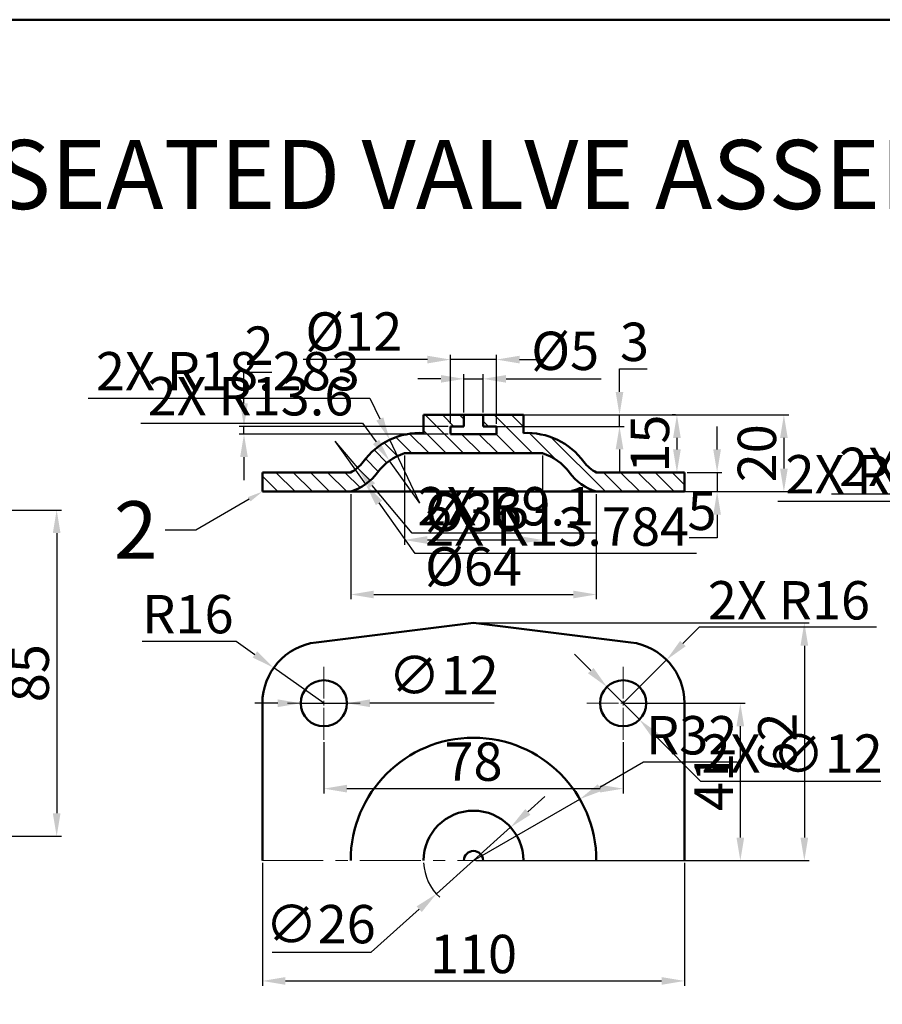
# Model space of a CAD drawing. Units: millimetres. Extents: x 147 to 984, y -369 to 435.
# Tile 7 of 10: x 475 to 699, y 179 to 435. Entities that reach past the tile are written whole.
import ezdxf
from ezdxf import colors
from ezdxf.entities.mleader import LeaderData, LeaderLine
from ezdxf.math import Vec2, Vec3

# ---------------------------------------------------------------- set-up
doc = ezdxf.new("R2010")
doc.units = ezdxf.units.MM
doc.header["$LTSCALE"] = 0.5
doc.linetypes.add('CENTER', pattern=[50.8, 31.75, -6.35, 6.35, -6.35])
for name, color, linetype, lineweight in [('M-CNTR', 1, 'CENTER', 18), ('M-DIMS', 2, 'Continuous', 25), ('M-HATC', 8, 'Continuous', 18), ('M-OUTL', 7, 'Continuous', 50), ('M-TEXT', 7, 'Continuous', 25)]:
    doc.layers.add(name, color=color, linetype=linetype, lineweight=lineweight)
doc.styles.get("Standard").update_dxf_attribs({"font": 'arial.ttf'})
doc.dimstyles.new('ISO-25', dxfattribs={"dimtxt": 10, "dimasz": 6, "dimexe": 1.25, "dimexo": 0.625, "dimtad": 1, "dimtoh": 1, "dimdec": 0, "dimtxsty": 'Standard', "dimcen": 2.5, "dimadec": 0, "dimazin": 0, "dimtfac": 1, "dimtdec": 0, "dimtmove": 0, "dimatfit": 3, "dimfxl": 1, "dimarcsym": 0})

# ---------------------------------------------------------------- blocks, each defined once
blk = doc.blocks.new('*D2')
at = {"layer": 'Defpoints', "color": 0, "transparency": 16777216}
for p in [(439.82, 307.49), (439.82, 222.49), (484.37, 222.49)]:
    blk.add_point(p, dxfattribs=at)
at = {"layer": 'M-DIMS', "color": 0, "lineweight": -2, "transparency": 16777216}
for p, q in [((440.44, 307.49), (485.62, 307.49)), ((484.37, 301.49), (484.37, 228.49)), ((440.44, 222.49), (485.62, 222.49))]:
    blk.add_line(p, q, dxfattribs=at)
at = {"layer": 'M-DIMS', "color": 0, "transparency": 16777216}
for points in [[(483.37, 301.49), (485.37, 301.49), (484.37, 307.49)], [(483.37, 228.49), (485.37, 228.49), (484.37, 222.49)]]:
    blk.add_solid(points, dxfattribs=at)
at = {"layer": 'M-DIMS', "color": 0, "transparency": 16777216, "insert": (478.64, 264.99), "char_height": 10, "attachment_point": 5, "rotation": 90}
blk.add_mtext('85', dxfattribs=at)
blk = doc.blocks.new('*U27')
at = {"layer": 'M-CNTR', "color": 0, "transparency": 16777216}
for p, q in [((0, 1.2), (0, 9.5)), ((-9.5, 0), (-1.2, 0)), ((1.2, 0), (9.5, 0)), ((0, -9.5), (0, -1.2))]:
    blk.add_line(p, q, dxfattribs=at)
at = {"layer": 'M-CNTR', "color": 0, "linetype": 'Continuous', "transparency": 16777216}
for p, q in [((-0.6, 0), (0.6, 0)), ((0, -0.6), (0, 0.6))]:
    blk.add_line(p, q, dxfattribs=at)
blk = doc.blocks.new('*U28')
at = {"layer": 'M-CNTR', "color": 0, "transparency": 16777216}
for p, q in [((0, 1.2), (0, 9.5)), ((-9.5, 0), (-1.2, 0)), ((1.2, 0), (9.5, 0)), ((0, -9.5), (0, -1.2))]:
    blk.add_line(p, q, dxfattribs=at)
at = {"layer": 'M-CNTR', "color": 0, "linetype": 'Continuous', "transparency": 16777216}
for p, q in [((-0.6, 0), (0.6, 0)), ((0, -0.6), (0, 0.6))]:
    blk.add_line(p, q, dxfattribs=at)
blk = doc.blocks.new('*D29')
at = {"layer": 'Defpoints', "color": 0, "transparency": 16777216}
for p in [(595.47, 341.7), (590.47, 332.31), (595.47, 332.31)]:
    blk.add_point(p, dxfattribs=at)
at = {"layer": 'M-DIMS', "color": 0, "lineweight": -2, "transparency": 16777216}
for p, q in [((584.47, 341.7), (578.47, 341.7)), ((590.47, 332.94), (590.47, 342.95)), ((590.47, 341.7), (595.47, 341.7)), ((595.47, 332.94), (595.47, 342.95)), ((601.47, 341.7), (626.23, 341.7))]:
    blk.add_line(p, q, dxfattribs=at)
at = {"layer": 'M-DIMS', "color": 0, "transparency": 16777216}
for points in [[(584.47, 342.7), (584.47, 340.7), (590.47, 341.7)], [(601.47, 342.7), (601.47, 340.7), (595.47, 341.7)]]:
    blk.add_solid(points, dxfattribs=at)
at = {"layer": 'M-DIMS', "color": 0, "transparency": 16777216, "insert": (616.85, 347.71), "char_height": 10, "attachment_point": 5}
blk.add_mtext('%%C5', dxfattribs=at)
blk = doc.blocks.new('*D30')
at = {"layer": 'Defpoints', "color": 0, "transparency": 16777216}
for p in [(598.97, 346.73), (586.97, 329.31), (598.97, 329.31)]:
    blk.add_point(p, dxfattribs=at)
at = {"layer": 'M-DIMS', "color": 0, "lineweight": -2, "transparency": 16777216}
for p, q in [((580.97, 346.73), (548.62, 346.73)), ((586.97, 329.94), (586.97, 347.98)), ((598.97, 346.73), (586.97, 346.73)), ((598.97, 329.94), (598.97, 347.98)), ((604.97, 346.73), (610.97, 346.73))]:
    blk.add_line(p, q, dxfattribs=at)
at = {"layer": 'M-DIMS', "color": 0, "transparency": 16777216}
for points in [[(580.97, 347.73), (580.97, 345.73), (586.97, 346.73)], [(604.97, 347.73), (604.97, 345.73), (598.97, 346.73)]]:
    blk.add_solid(points, dxfattribs=at)
at = {"layer": 'M-DIMS', "color": 0, "transparency": 16777216, "insert": (561.79, 352.74), "char_height": 10, "attachment_point": 5}
blk.add_mtext('%%C12', dxfattribs=at)
blk = doc.blocks.new('*D31')
at = {"layer": 'Defpoints', "color": 0, "transparency": 16777216}
for p in [(595.47, 332.31), (595.47, 329.31), (631.01, 329.31)]:
    blk.add_point(p, dxfattribs=at)
at = {"layer": 'M-DIMS', "color": 0, "lineweight": -2, "transparency": 16777216}
for p, q in [((631.01, 338.31), (631.01, 344.31)), ((631.01, 344.31), (638.18, 344.31)), ((596.1, 332.31), (632.26, 332.31)), ((631.01, 329.31), (631.01, 332.31)), ((596.1, 329.31), (632.26, 329.31)), ((631.01, 323.31), (631.01, 317.31))]:
    blk.add_line(p, q, dxfattribs=at)
at = {"layer": 'M-DIMS', "color": 0, "transparency": 16777216}
for points in [[(630.01, 338.31), (632.01, 338.31), (631.01, 332.31)], [(630.01, 323.31), (632.01, 323.31), (631.01, 329.31)]]:
    blk.add_solid(points, dxfattribs=at)
at = {"layer": 'M-DIMS', "color": 0, "transparency": 16777216, "insert": (634.91, 350.05), "char_height": 10, "attachment_point": 5}
blk.add_mtext('3', dxfattribs=at)
blk = doc.blocks.new('*D32')
at = {"layer": 'Defpoints', "color": 0, "transparency": 16777216}
for p in [(586.97, 329.31), (533.17, 327.31), (586.97, 327.31)]:
    blk.add_point(p, dxfattribs=at)
at = {"layer": 'M-DIMS', "color": 0, "lineweight": -2, "transparency": 16777216}
for p, q in [((533.17, 335.31), (533.17, 343.41)), ((533.17, 343.41), (540.42, 343.41)), ((586.35, 329.31), (531.92, 329.31)), ((533.17, 327.31), (533.17, 329.31)), ((586.35, 327.31), (531.92, 327.31)), ((533.17, 321.31), (533.17, 315.31))]:
    blk.add_line(p, q, dxfattribs=at)
at = {"layer": 'M-DIMS', "color": 0, "transparency": 16777216}
for points in [[(532.17, 335.31), (534.17, 335.31), (533.17, 329.31)], [(532.17, 321.31), (534.17, 321.31), (533.17, 327.31)]]:
    blk.add_solid(points, dxfattribs=at)
at = {"layer": 'M-DIMS', "color": 0, "transparency": 16777216, "insert": (537.11, 349.06), "char_height": 10, "attachment_point": 5}
blk.add_mtext('2', dxfattribs=at)
blk = doc.blocks.new('*D33')
at = {"layer": 'Defpoints', "color": 0, "transparency": 16777216}
for p in [(560.97, 312.31), (624.97, 312.31), (624.97, 285.51)]:
    blk.add_point(p, dxfattribs=at)
at = {"layer": 'M-DIMS', "color": 0, "lineweight": -2, "transparency": 16777216}
for p, q in [((560.97, 311.69), (560.97, 284.26)), ((624.97, 311.69), (624.97, 284.26)), ((566.97, 285.51), (618.97, 285.51))]:
    blk.add_line(p, q, dxfattribs=at)
at = {"layer": 'M-DIMS', "color": 0, "transparency": 16777216}
for points in [[(566.97, 286.51), (566.97, 284.51), (560.97, 285.51)], [(618.97, 286.51), (618.97, 284.51), (624.97, 285.51)]]:
    blk.add_solid(points, dxfattribs=at)
at = {"layer": 'M-DIMS', "color": 0, "transparency": 16777216, "insert": (592.97, 291.52), "char_height": 10, "attachment_point": 5}
blk.add_mtext('%%C64', dxfattribs=at)
blk = doc.blocks.new('*D34')
at = {"layer": 'Defpoints', "color": 0, "transparency": 16777216}
for p in [(574.97, 322.31), (610.97, 322.31), (610.97, 299.71)]:
    blk.add_point(p, dxfattribs=at)
at = {"layer": 'M-DIMS', "color": 0, "lineweight": -2, "transparency": 16777216}
for p, q in [((574.97, 321.69), (574.97, 298.46)), ((610.97, 321.69), (610.97, 298.46)), ((580.97, 299.71), (604.97, 299.71))]:
    blk.add_line(p, q, dxfattribs=at)
at = {"layer": 'M-DIMS', "color": 0, "transparency": 16777216}
for points in [[(580.97, 300.71), (580.97, 298.71), (574.97, 299.71)], [(604.97, 300.71), (604.97, 298.71), (610.97, 299.71)]]:
    blk.add_solid(points, dxfattribs=at)
at = {"layer": 'M-DIMS', "color": 0, "transparency": 16777216, "insert": (592.97, 305.72), "char_height": 10, "attachment_point": 5}
blk.add_mtext('%%C36', dxfattribs=at)
blk = doc.blocks.new('*D35')
at = {"layer": 'Defpoints', "color": 0, "transparency": 16777216}
for p in [(593.07, 332.31), (592.97, 312.31), (673.84, 312.31)]:
    blk.add_point(p, dxfattribs=at)
at = {"layer": 'M-DIMS', "color": 0, "lineweight": -2, "transparency": 16777216}
for p, q in [((593.69, 332.31), (675.09, 332.31)), ((673.84, 326.31), (673.84, 318.31)), ((593.6, 312.31), (675.09, 312.31))]:
    blk.add_line(p, q, dxfattribs=at)
at = {"layer": 'M-DIMS', "color": 0, "transparency": 16777216}
for points in [[(672.84, 326.31), (674.84, 326.31), (673.84, 332.31)], [(672.84, 318.31), (674.84, 318.31), (673.84, 312.31)]]:
    blk.add_solid(points, dxfattribs=at)
at = {"layer": 'M-DIMS', "color": 0, "transparency": 16777216, "insert": (668.1, 322.31), "char_height": 10, "attachment_point": 5, "rotation": 90}
blk.add_mtext('20', dxfattribs=at)
blk = doc.blocks.new('*D36')
at = {"layer": 'Defpoints', "color": 0, "transparency": 16777216}
for p in [(647.97, 317.31), (647.97, 312.31), (656.44, 312.31)]:
    blk.add_point(p, dxfattribs=at)
at = {"layer": 'M-DIMS', "color": 0, "lineweight": -2, "transparency": 16777216}
for p, q in [((656.44, 323.31), (656.44, 329.31)), ((648.6, 317.31), (657.69, 317.31)), ((656.44, 317.31), (656.44, 312.31)), ((648.6, 312.31), (657.69, 312.31)), ((656.44, 306.31), (656.44, 300.31)), ((656.44, 300.31), (649.19, 300.31))]:
    blk.add_line(p, q, dxfattribs=at)
at = {"layer": 'M-DIMS', "color": 0, "transparency": 16777216}
for points in [[(655.44, 323.31), (657.44, 323.31), (656.44, 317.31)], [(655.44, 306.31), (657.44, 306.31), (656.44, 312.31)]]:
    blk.add_solid(points, dxfattribs=at)
at = {"layer": 'M-DIMS', "color": 0, "transparency": 16777216, "insert": (652.5, 306.02), "char_height": 10, "attachment_point": 5}
blk.add_mtext('5', dxfattribs=at)
blk = doc.blocks.new('*D37')
at = {"layer": 'Defpoints', "color": 0, "transparency": 16777216}
for p in [(646.27, 332.31), (645.97, 317.31), (646.27, 317.31)]:
    blk.add_point(p, dxfattribs=at)
at = {"layer": 'M-DIMS', "color": 0, "lineweight": -2, "transparency": 16777216}
for p, q in [((645.64, 332.31), (644.72, 332.31)), ((645.97, 326.31), (645.97, 323.31)), ((645.64, 317.31), (644.72, 317.31))]:
    blk.add_line(p, q, dxfattribs=at)
at = {"layer": 'M-DIMS', "color": 0, "transparency": 16777216}
for points in [[(644.97, 326.31), (646.97, 326.31), (645.97, 332.31)], [(644.97, 323.31), (646.97, 323.31), (645.97, 317.31)]]:
    blk.add_solid(points, dxfattribs=at)
at = {"layer": 'M-DIMS', "color": 0, "transparency": 16777216, "insert": (640.24, 324.81), "char_height": 10, "attachment_point": 5, "rotation": 90}
blk.add_mtext('15', dxfattribs=at)
blk = doc.blocks.new('*D38')
at = {"layer": 'Defpoints', "color": 0, "transparency": 16777216}
for p in [(540.92, 266.42), (553.97, 257.16)]:
    blk.add_point(p, dxfattribs=at)
at = {"layer": 'M-DIMS', "color": 0, "lineweight": -2, "transparency": 16777216}
for p, q in [((506.62, 273.36), (531.13, 273.36)), ((531.13, 273.36), (536.03, 269.89)), ((553.97, 257.16), (540.92, 266.42))]:
    blk.add_line(p, q, dxfattribs=at)
at = {"layer": 'M-DIMS', "color": 0, "transparency": 16777216}
blk.add_solid([(536.61, 270.71), (535.45, 269.07), (540.92, 266.42)], dxfattribs=at)
at = {"layer": 'M-DIMS', "color": 0, "transparency": 16777216, "insert": (518.56, 279.09), "char_height": 10, "attachment_point": 5}
blk.add_mtext('R16', dxfattribs=at)
blk = doc.blocks.new('*D39')
at = {"layer": 'Defpoints', "color": 0, "transparency": 16777216}
for p in [(602.65, 224.84), (583.29, 207.48)]:
    blk.add_point(p, dxfattribs=at)
at = {"layer": 'M-DIMS', "color": 0, "lineweight": -2, "transparency": 16777216}
for p, q in [((607.12, 228.84), (611.59, 232.85)), ((602.65, 224.84), (583.29, 207.48)), ((566.33, 192.29), (578.82, 203.48)), ((540.51, 192.29), (566.33, 192.29))]:
    blk.add_line(p, q, dxfattribs=at)
blk.add_arc((592.97, 216.16), 13, 182.7546, 227.3746, dxfattribs=at)
at = {"layer": 'M-DIMS', "color": 0, "transparency": 16777216}
for points in [[(606.45, 229.59), (607.79, 228.1), (602.65, 224.84)], [(578.15, 204.23), (579.49, 202.74), (583.29, 207.48)]]:
    blk.add_solid(points, dxfattribs=at)
at = {"layer": 'M-DIMS', "color": 0, "transparency": 16777216, "insert": (553.11, 198.3), "char_height": 10, "attachment_point": 5}
blk.add_mtext('∅26', dxfattribs=at)
blk = doc.blocks.new('*D40')
at = {"layer": 'Defpoints', "color": 0, "transparency": 16777216}
for p in [(547.97, 257.16), (559.97, 257.16)]:
    blk.add_point(p, dxfattribs=at)
at = {"layer": 'M-DIMS', "color": 0, "lineweight": -2, "transparency": 16777216}
for p, q in [((541.97, 257.16), (535.97, 257.16)), ((547.97, 257.16), (559.97, 257.16)), ((598.32, 257.16), (565.97, 257.16))]:
    blk.add_line(p, q, dxfattribs=at)
at = {"layer": 'M-DIMS', "color": 0, "transparency": 16777216}
for points in [[(541.97, 258.16), (541.97, 256.16), (547.97, 257.16)], [(565.97, 258.16), (565.97, 256.16), (559.97, 257.16)]]:
    blk.add_solid(points, dxfattribs=at)
at = {"layer": 'M-DIMS', "color": 0, "transparency": 16777216, "insert": (585.15, 263.17), "char_height": 10, "attachment_point": 5}
blk.add_mtext('∅12', dxfattribs=at)
blk = doc.blocks.new('*D41')
at = {"layer": 'Defpoints', "color": 0, "transparency": 16777216}
for p in [(553.97, 247.66), (631.97, 247.66), (631.97, 234.91)]:
    blk.add_point(p, dxfattribs=at)
at = {"layer": 'M-DIMS', "color": 0, "lineweight": -2, "transparency": 16777216}
for p, q in [((553.97, 247.04), (553.97, 233.66)), ((631.97, 247.04), (631.97, 233.66)), ((559.97, 234.91), (625.97, 234.91))]:
    blk.add_line(p, q, dxfattribs=at)
at = {"layer": 'M-DIMS', "color": 0, "transparency": 16777216}
for points in [[(559.97, 235.91), (559.97, 233.91), (553.97, 234.91)], [(625.97, 235.91), (625.97, 233.91), (631.97, 234.91)]]:
    blk.add_solid(points, dxfattribs=at)
at = {"layer": 'M-DIMS', "color": 0, "transparency": 16777216, "insert": (592.97, 240.65), "char_height": 10, "attachment_point": 5}
blk.add_mtext('78', dxfattribs=at)
blk = doc.blocks.new('*D42')
at = {"layer": 'Defpoints', "color": 0, "transparency": 16777216}
for p in [(537.97, 216.16), (647.97, 216.16), (647.97, 184.79)]:
    blk.add_point(p, dxfattribs=at)
at = {"layer": 'M-DIMS', "color": 0, "lineweight": -2, "transparency": 16777216}
for p, q in [((537.97, 215.54), (537.97, 183.54)), ((647.97, 215.54), (647.97, 183.54)), ((543.97, 184.79), (641.97, 184.79))]:
    blk.add_line(p, q, dxfattribs=at)
at = {"layer": 'M-DIMS', "color": 0, "transparency": 16777216}
for points in [[(543.97, 185.79), (543.97, 183.79), (537.97, 184.79)], [(641.97, 185.79), (641.97, 183.79), (647.97, 184.79)]]:
    blk.add_solid(points, dxfattribs=at)
at = {"layer": 'M-DIMS', "color": 0, "transparency": 16777216, "insert": (592.97, 190.52), "char_height": 10, "attachment_point": 5}
blk.add_mtext('110', dxfattribs=at)
blk = doc.blocks.new('*D43')
at = {"layer": 'Defpoints', "color": 0, "transparency": 16777216}
for p in [(592.97, 278.16), (592.97, 216.16), (679.17, 216.16)]:
    blk.add_point(p, dxfattribs=at)
at = {"layer": 'M-DIMS', "color": 0, "lineweight": -2, "transparency": 16777216}
for p, q in [((593.6, 278.16), (680.42, 278.16)), ((679.17, 272.16), (679.17, 222.16)), ((593.6, 216.16), (680.42, 216.16))]:
    blk.add_line(p, q, dxfattribs=at)
at = {"layer": 'M-DIMS', "color": 0, "transparency": 16777216}
for points in [[(678.17, 272.16), (680.17, 272.16), (679.17, 278.16)], [(678.17, 222.16), (680.17, 222.16), (679.17, 216.16)]]:
    blk.add_solid(points, dxfattribs=at)
at = {"layer": 'M-DIMS', "color": 0, "transparency": 16777216, "insert": (673.44, 247.16), "char_height": 10, "attachment_point": 5, "rotation": 90}
blk.add_mtext('62', dxfattribs=at)
blk = doc.blocks.new('*D44')
at = {"layer": 'Defpoints', "color": 0, "transparency": 16777216}
for p in [(631.97, 257.16), (631.97, 216.16), (662.49, 216.16)]:
    blk.add_point(p, dxfattribs=at)
at = {"layer": 'M-DIMS', "color": 0, "lineweight": -2, "transparency": 16777216}
for p, q in [((632.6, 257.16), (663.74, 257.16)), ((662.49, 251.16), (662.49, 222.16)), ((632.6, 216.16), (663.74, 216.16))]:
    blk.add_line(p, q, dxfattribs=at)
at = {"layer": 'M-DIMS', "color": 0, "transparency": 16777216}
for points in [[(661.49, 251.16), (663.49, 251.16), (662.49, 257.16)], [(661.49, 222.16), (663.49, 222.16), (662.49, 216.16)]]:
    blk.add_solid(points, dxfattribs=at)
at = {"layer": 'M-DIMS', "color": 0, "transparency": 16777216, "insert": (656.84, 236.66), "char_height": 10, "attachment_point": 5, "rotation": 90}
blk.add_mtext('41', dxfattribs=at)
blk = doc.blocks.new('*D161')
at = {"layer": 'Defpoints', "color": 0, "ltscale": 0.5, "transparency": 16777216}
for p in [(643.28, 268.48), (631.97, 257.16)]:
    blk.add_point(p, dxfattribs=at)
at = {"layer": 'M-DIMS', "color": 0, "lineweight": -2, "ltscale": 0.5, "transparency": 16777216}
for p, q in [((651.76, 276.97), (647.52, 272.72)), ((697.93, 276.97), (651.76, 276.97)), ((631.97, 257.16), (643.28, 268.48))]:
    blk.add_line(p, q, dxfattribs=at)
at = {"layer": 'M-DIMS', "color": 0, "ltscale": 0.5, "transparency": 16777216}
blk.add_solid([(646.81, 273.43), (648.23, 272.02), (643.28, 268.48)], dxfattribs=at)
at = {"layer": 'M-DIMS', "color": 0, "ltscale": 0.5, "transparency": 16777216, "insert": (675.16, 282.7), "char_height": 10, "attachment_point": 5}
blk.add_mtext('2X R16', dxfattribs=at)
blk = doc.blocks.new('*D162')
at = {"layer": 'Defpoints', "color": 0, "ltscale": 0.5, "transparency": 16777216}
for p in [(627.74, 261.42), (636.2, 252.9)]:
    blk.add_point(p, dxfattribs=at)
at = {"layer": 'M-DIMS', "color": 0, "lineweight": -2, "ltscale": 0.5, "transparency": 16777216}
for p, q in [((623.52, 265.68), (619.29, 269.94)), ((627.74, 261.42), (636.2, 252.9)), ((652.24, 236.74), (640.42, 248.64)), ((699.09, 236.74), (652.24, 236.74))]:
    blk.add_line(p, q, dxfattribs=at)
at = {"layer": 'M-DIMS', "color": 0, "ltscale": 0.5, "transparency": 16777216}
for points in [[(624.23, 266.38), (622.81, 264.97), (627.74, 261.42)], [(641.13, 249.35), (639.71, 247.94), (636.2, 252.9)]]:
    blk.add_solid(points, dxfattribs=at)
at = {"layer": 'M-DIMS', "color": 0, "ltscale": 0.5, "transparency": 16777216, "insert": (675.98, 242.75), "char_height": 10, "attachment_point": 5}
blk.add_mtext('2X ∅12', dxfattribs=at)
blk = doc.blocks.new('*D163')
at = {"layer": 'Defpoints', "color": 0, "ltscale": 0.5, "transparency": 16777216}
for p in [(620.67, 232.18), (592.97, 216.16)]:
    blk.add_point(p, dxfattribs=at)
at = {"layer": 'M-DIMS', "color": 0, "lineweight": -2, "ltscale": 0.5, "transparency": 16777216}
for p, q in [((637.29, 241.8), (625.86, 235.19)), ((661.71, 241.8), (637.29, 241.8)), ((592.97, 216.16), (620.67, 232.18))]:
    blk.add_line(p, q, dxfattribs=at)
at = {"layer": 'M-DIMS', "color": 0, "ltscale": 0.5, "transparency": 16777216}
blk.add_solid([(625.36, 236.05), (626.36, 234.32), (620.67, 232.18)], dxfattribs=at)
at = {"layer": 'M-DIMS', "color": 0, "ltscale": 0.5, "transparency": 16777216, "insert": (649.81, 247.53), "char_height": 10, "attachment_point": 5}
blk.add_mtext('R32', dxfattribs=at)
blk = doc.blocks.new('*D164')
at = {"layer": 'Defpoints', "color": 0, "ltscale": 0.5, "transparency": 16777216}
for p in [(571.13, 325.83), (578.97, 309.31)]:
    blk.add_point(p, dxfattribs=at)
at = {"layer": 'M-DIMS', "color": 0, "lineweight": -2, "ltscale": 0.5, "transparency": 16777216}
for p, q in [((492.61, 336.67), (565.98, 336.67)), ((565.98, 336.67), (568.55, 331.25)), ((578.97, 309.31), (571.13, 325.83))]:
    blk.add_line(p, q, dxfattribs=at)
at = {"layer": 'M-DIMS', "color": 0, "ltscale": 0.5, "transparency": 16777216}
blk.add_solid([(569.46, 331.68), (567.65, 330.82), (571.13, 325.83)], dxfattribs=at)
at = {"layer": 'M-DIMS', "color": 0, "ltscale": 0.5, "transparency": 16777216, "insert": (528.98, 342.4), "char_height": 10, "attachment_point": 5}
blk.add_mtext('2X R18.283', dxfattribs=at)
blk = doc.blocks.new('*D165')
at = {"layer": 'Defpoints', "color": 0, "ltscale": 0.5, "transparency": 16777216}
for p in [(556.86, 325.47), (564.87, 314.25)]:
    blk.add_point(p, dxfattribs=at)
at = {"layer": 'M-DIMS', "color": 0, "lineweight": -2, "ltscale": 0.5, "transparency": 16777216}
for p, q in [((556.86, 325.47), (564.87, 314.25)), ((577.78, 296.17), (568.36, 309.37)), ((651.11, 296.17), (577.78, 296.17))]:
    blk.add_line(p, q, dxfattribs=at)
at = {"layer": 'M-DIMS', "color": 0, "ltscale": 0.5, "transparency": 16777216}
blk.add_solid([(569.17, 309.95), (567.54, 308.79), (564.87, 314.25)], dxfattribs=at)
at = {"layer": 'M-DIMS', "color": 0, "ltscale": 0.5, "transparency": 16777216, "insert": (614.76, 301.91), "char_height": 10, "attachment_point": 5}
blk.add_mtext('2X R13.784', dxfattribs=at)
blk = doc.blocks.new('*D166')
at = {"layer": 'Defpoints', "color": 0, "ltscale": 0.5, "transparency": 16777216}
for p in [(571.06, 320.38), (578.97, 309.31)]:
    blk.add_point(p, dxfattribs=at)
at = {"layer": 'M-DIMS', "color": 0, "lineweight": -2, "ltscale": 0.5, "transparency": 16777216}
for p, q in [((506.27, 330.15), (564.09, 330.15)), ((564.09, 330.15), (567.58, 325.26)), ((578.97, 309.31), (571.06, 320.38))]:
    blk.add_line(p, q, dxfattribs=at)
at = {"layer": 'M-DIMS', "color": 0, "ltscale": 0.5, "transparency": 16777216}
blk.add_solid([(568.39, 325.84), (566.76, 324.68), (571.06, 320.38)], dxfattribs=at)
at = {"layer": 'M-DIMS', "color": 0, "ltscale": 0.5, "transparency": 16777216, "insert": (534.87, 335.88), "char_height": 10, "attachment_point": 5}
blk.add_mtext('2X R13.6', dxfattribs=at)
blk = doc.blocks.new('*D167')
at = {"layer": 'Defpoints', "color": 0, "ltscale": 0.5, "transparency": 16777216}
for p in [(556.86, 325.47), (562.71, 318.5)]:
    blk.add_point(p, dxfattribs=at)
at = {"layer": 'M-DIMS', "color": 0, "lineweight": -2, "ltscale": 0.5, "transparency": 16777216}
for p, q in [((556.86, 325.47), (562.71, 318.5)), ((576.98, 301.48), (566.56, 313.9)), ((625.11, 301.48), (576.98, 301.48))]:
    blk.add_line(p, q, dxfattribs=at)
at = {"layer": 'M-DIMS', "color": 0, "ltscale": 0.5, "transparency": 16777216}
blk.add_solid([(567.33, 314.54), (565.8, 313.26), (562.71, 318.5)], dxfattribs=at)
at = {"layer": 'M-DIMS', "color": 0, "ltscale": 0.5, "transparency": 16777216, "insert": (601.36, 307.21), "char_height": 10, "attachment_point": 5}
blk.add_mtext('2X R9.1', dxfattribs=at)
blk = doc.blocks.new('*D168')
at = {"layer": 'Defpoints', "color": 0, "ltscale": 0.5, "transparency": 16777216}
for p in [(761.78, 299.23), (788.72, 281.61)]:
    blk.add_point(p, dxfattribs=at)
at = {"layer": 'M-DIMS', "color": 0, "lineweight": -2, "ltscale": 0.5, "transparency": 16777216}
for p, q in [((672.29, 309.8), (745.62, 309.8)), ((745.62, 309.8), (756.76, 302.52)), ((788.72, 281.61), (761.78, 299.23))]:
    blk.add_line(p, q, dxfattribs=at)
at = {"layer": 'M-DIMS', "color": 0, "ltscale": 0.5, "transparency": 16777216}
blk.add_solid([(757.31, 303.35), (756.21, 301.68), (761.78, 299.23)], dxfattribs=at)
at = {"layer": 'M-DIMS', "color": 0, "ltscale": 0.5, "transparency": 16777216, "insert": (708.64, 315.54), "char_height": 10, "attachment_point": 5}
blk.add_mtext('2X R32.194', dxfattribs=at)
blk = doc.blocks.new('*D169')
at = {"layer": 'Defpoints', "color": 0, "ltscale": 0.5, "transparency": 16777216}
for p in [(770.53, 300.44), (788.72, 281.61)]:
    blk.add_point(p, dxfattribs=at)
at = {"layer": 'M-DIMS', "color": 0, "lineweight": -2, "ltscale": 0.5, "transparency": 16777216}
for p, q in [((686.24, 311.74), (759.61, 311.74)), ((759.61, 311.74), (766.36, 304.76)), ((788.72, 281.61), (770.53, 300.44))]:
    blk.add_line(p, q, dxfattribs=at)
at = {"layer": 'M-DIMS', "color": 0, "ltscale": 0.5, "transparency": 16777216}
blk.add_solid([(767.08, 305.45), (765.64, 304.06), (770.53, 300.44)], dxfattribs=at)
at = {"layer": 'M-DIMS', "color": 0, "ltscale": 0.5, "transparency": 16777216, "insert": (722.61, 317.47), "char_height": 10, "attachment_point": 5}
blk.add_mtext('2X R26.187', dxfattribs=at)

msp = doc.modelspace()

# ---------------------------------------------------------------- hatches: boundary and pattern name
at = {"layer": 'M-HATC'}
h = msp.add_hatch(dxfattribs=at)
h.set_pattern_fill('ANSI31', color=256, angle=90)
h.set_pattern_definition([(135, (-50.2943, 29.0374), (-2.245064, -2.245064), [])])
h.paths.add_polyline_path([(560.9704, 312.3118, 0.16001287), (567.9704, 317.3118, -0.16230755), (574.9704, 322.3118), (610.9704, 322.3118, -0.16230755), (617.9704, 317.3118, 0.16001287), (624.9704, 312.3118), (647.9704, 312.3118), (647.9704, 317.3118), (625.0469, 317.3118, -0.12147977), (621.7173, 320.1231, 0.25348697), (605.9704, 327.5694), (605.9704, 332.3118), (595.4704, 332.3118), (595.4704, 329.3118), (598.9704, 329.3118), (598.9704, 327.3118), (586.9704, 327.3118), (586.9704, 329.3118), (590.4704, 329.3118), (590.4704, 332.3118), (579.9704, 332.3118), (579.9704, 327.5694, 0.25348697), (564.2234, 320.1231, -0.12147977), (560.8939, 317.3118), (537.9704, 317.3118), (537.9704, 312.3118)])

# ---------------------------------------------------------------- linework, layer by layer
at = {"layer": 'M-CNTR'}
msp.add_line((537.9704, 216.1607), (647.9704, 216.1607), dxfattribs=at)
at = {"layer": 'M-OUTL'}
for p, q in [((592.9704, 332.3118), (579.9704, 332.3118)), ((579.9704, 332.3118), (579.9704, 327.5694)), ((592.9704, 332.3118), (590.4704, 332.3118)), ((590.4704, 332.3118), (590.4704, 329.3118)), ((592.9704, 332.3118), (605.9704, 332.3118)), ((592.9704, 332.3118), (595.4704, 332.3118)), ((595.4704, 332.3118), (595.4704, 329.3118)), ((605.9704, 332.3118), (605.9704, 327.5694)), ((586.9704, 329.3118), (586.9704, 327.3118)), ((590.4704, 329.3118), (586.9704, 329.3118)), ((598.9704, 329.3118), (595.4704, 329.3118)), ((598.9704, 327.3118), (598.9704, 329.3118)), ((586.9704, 327.3118), (598.9704, 327.3118)), ((574.9704, 322.3118), (610.9704, 322.3118)), ((537.9704, 317.3118), (537.9704, 312.3118)), ((560.9704, 317.3118), (537.9704, 317.3118)), ((647.9704, 317.3118), (624.9704, 317.3118)), ((647.9704, 312.3118), (647.9704, 317.3118)), ((537.9704, 312.3118), (647.9704, 312.3118)), ((551.9856, 273.0371), (592.9704, 278.1607)), ((592.9704, 278.1607), (633.9551, 273.0371)), ((537.9704, 257.1607), (537.9704, 216.1607)), ((647.9704, 216.1607), (647.9704, 257.1607))]:
    msp.add_line(p, q, dxfattribs=at)
at = {"layer": 'M-OUTL', "ltscale": 0.5}
msp.add_lwpolyline([(147.3511, 435.3078), (984.0884, 435.3078), (984.0884, -369.4968), (147.3511, -369.4968)], close=True, dxfattribs=at)
at = {"layer": 'M-OUTL'}
for points in [[(579.9704, 327.5694, 0.25432677), (564.1894, 320.0765, -0.11987163), (560.8939, 317.3118, -0.11987163)], [(605.9704, 327.5694, -0.25432677), (621.7514, 320.0765, 0.11987163), (625.0469, 317.3118, 0.11987163)], [(574.9704, 322.3118, 0.16230755), (567.9704, 317.3118, -0.16001287), (560.9704, 312.3118)]]:
    msp.add_lwpolyline(points, format="xyb", dxfattribs=at)
for centre in [(553.9704, 257.1607), (631.9704, 257.1607)]:
    msp.add_circle(centre, 6, dxfattribs=at)
for centre, radius, start, end in [((606.9718, 309.3138), 13.5991, 36.024036, 72.900608), ((629.0822, 325.4684), 13.7842, 216.025769, 252.644314), ((553.9704, 257.1607), 16, 97.125683, 180), ((631.9704, 257.1607), 16, 0, 82.874317), ((592.9704, 216.1607), 32, 0, 180), ((592.9704, 216.1607), 13, 0, 180), ((592.9704, 216.1607), 2.5, 0, 180)]:
    msp.add_arc(centre, radius, start, end, dxfattribs=at)

# ---------------------------------------------------------------- block references
at = {"layer": 'M-CNTR'}
for name, p in [('*U28', (553.9704, 257.1607)), ('*U27', (631.9704, 257.1607))]:
    msp.add_blockref(name, p, dxfattribs=at)

# ---------------------------------------------------------------- texts
at = {"layer": 'M-TEXT', "ltscale": 0.5, "insert": (313.9939, 403.9552), "char_height": 18, "attachment_point": 1}
msp.add_mtext_dynamic_manual_height_columns('\\pxqc;RUBBER-SEATED VALVE ASSEMBLY', width=497.441574, gutter_width=12.5, heights=[0], dxfattribs=at)

# ---------------------------------------------------------------- dimensions: what is measured, and where the dimension line sits
at = {"layer": 'M-DIMS'}
for base, p1, p2, picture, middle in [((598.9704, 346.7319), (586.9704, 329.3118), (598.9704, 329.3118), '*D30', (561.7942, 346.7319)), ((624.9704, 285.511), (560.9704, 312.3118), (624.9704, 312.3118), '*D33', (592.9704, 285.511))]:
    dim = msp.add_linear_dim(base=base, p1=p1, p2=p2, text='%%C<>', dimstyle='ISO-25', override={"dimclrd": 0, "dimclre": 0, "dimclrt": 0}, dxfattribs=at)
    dim.commit()
    dim.dimension.update_dxf_attribs({"geometry": picture, "text_midpoint": middle, "dimtype": 160})
at = {"layer": 'M-DIMS', "ltscale": 0.5}
for center, mpoint, override, picture, middle in [((578.9689, 309.3138), (571.1271, 325.8297), {"dimdec": 3, "dimlfac": 1, "dimrnd": 0, "dimzin": 0, "dimdsep": 46, "dimlunit": 2}, '*D164', (528.9841, 342.404)), ((578.9689, 309.3138), (571.0649, 320.3801), {"dimdec": 1, "dimlfac": 1, "dimrnd": 0, "dimzin": 0, "dimdsep": 46, "dimlunit": 2}, '*D166', (534.8671, 335.8792)), ((556.8585, 325.4684), (564.8703, 314.2516), {"dimdec": 3, "dimlfac": 1, "dimrnd": 0, "dimzin": 0, "dimdsep": 46, "dimlunit": 2}, '*D165', (614.7598, 301.9058)), ((556.8585, 325.4684), (562.7073, 318.4966), {"dimdec": 1, "dimlfac": 1, "dimrnd": 0, "dimzin": 0, "dimdsep": 46, "dimlunit": 2}, '*D167', (601.3596, 307.2109)), ((631.9704, 257.1607), (643.2792, 268.4792), {"dimdec": 0, "dimlfac": 1, "dimrnd": 0, "dimzin": 0, "dimdsep": 46, "dimlunit": 2}, '*D161', (675.1587, 282.6989))]:
    dim = msp.add_radius_dim(center=center, mpoint=mpoint, text='2X <>', dimstyle='ISO-25', override=override, dxfattribs=at)
    dim.commit()
    dim.dimension.update_dxf_attribs({"geometry": picture, "text_midpoint": middle})
at = {"layer": 'M-DIMS'}
for base, p1, p2, picture, middle in [((533.173, 327.3118), (586.9704, 329.3118), (586.9704, 327.3118), '*D32', (537.1097, 343.4109)), ((631.0064, 329.3118), (595.4704, 332.3118), (595.4704, 329.3118), '*D31', (634.9057, 344.3118)), ((679.1676, 216.1607), (592.9704, 278.1607), (592.9704, 216.1607), '*D43', (679.1676, 247.1607)), ((662.4894, 216.1607), (631.9704, 257.1607), (631.9704, 216.1607), '*D44', (662.4894, 236.6607))]:
    dim = msp.add_linear_dim(base=base, p1=p1, p2=p2, angle=90, dimstyle='ISO-25', override={"dimclrd": 0, "dimclre": 0, "dimclrt": 0}, dxfattribs=at)
    dim.commit()
    dim.dimension.update_dxf_attribs({"geometry": picture, "text_midpoint": middle, "dimtype": 160})
for base, p1, p2, picture, middle in [((595.4704, 341.6992), (590.4704, 332.3118), (595.4704, 332.3118), '*D29', (616.8505, 347.7096)), ((610.9704, 299.7091), (574.9704, 322.3118), (610.9704, 322.3118), '*D34', (592.9704, 305.7195))]:
    dim = msp.add_linear_dim(base=base, p1=p1, p2=p2, text='%%C<>', dimstyle='ISO-25', override={"dimclrd": 0, "dimclre": 0, "dimclrt": 0}, dxfattribs=at)
    dim.commit()
    dim.dimension.update_dxf_attribs({"geometry": picture, "text_midpoint": middle})
for base, p1, p2, picture, middle in [((673.8353, 312.3118), (593.0685, 332.3118), (592.9704, 312.3118), '*D35', (668.1046, 322.3118)), ((645.9662, 317.3118), (646.269, 332.3118), (646.269, 317.3118), '*D37', (640.2355, 324.8118)), ((656.4431, 312.3118), (647.9704, 317.3118), (647.9704, 312.3118), '*D36', (652.5029, 306.022))]:
    dim = msp.add_linear_dim(base=base, p1=p1, p2=p2, angle=90, dimstyle='ISO-25', override={"dimclrd": 0, "dimclre": 0, "dimclrt": 0}, dxfattribs=at)
    dim.commit()
    dim.dimension.update_dxf_attribs({"geometry": picture, "text_midpoint": middle})
at = {"layer": 'M-DIMS', "ltscale": 0.5}
for mpoint, picture, middle in [((770.5262, 300.4408), '*D169', (722.6122, 311.7399)), ((761.7807, 299.2312), '*D168', (708.6398, 309.8046))]:
    dim = msp.add_radius_dim(center=(788.7228, 281.6089), mpoint=mpoint, text='2X <>', dimstyle='ISO-25', override={"dimdec": 3, "dimlfac": 1, "dimrnd": 0, "dimzin": 0, "dimdsep": 46, "dimlunit": 2}, dxfattribs=at)
    dim.commit()
    dim.dimension.update_dxf_attribs({"geometry": picture, "text_midpoint": middle, "dimtype": 164})
at = {"layer": 'M-DIMS'}
dim = msp.add_aligned_dim(p1=(439.8179, 307.4916), p2=(439.8179, 222.4916), distance=44.551, dimstyle='ISO-25', override={"dimclrd": 0, "dimclre": 0, "dimclrt": 0}, dxfattribs=at)
dim.commit()
dim.dimension.update_dxf_attribs({"geometry": '*D2', "text_midpoint": (478.6381, 264.9916)})
dim = msp.add_radius_dim(center=(553.9704, 257.1607), mpoint=(540.9204, 266.418), dimstyle='ISO-25', override={"dimclrd": 0, "dimclre": 0, "dimclrt": 0}, dxfattribs=at)
dim.commit()
dim.dimension.update_dxf_attribs({"geometry": '*D38', "text_midpoint": (518.5639, 279.0918)})
for p1, p2, picture, middle in [((547.9704, 257.1607), (559.9704, 257.1607), '*D40', (585.1465, 263.1711)), ((602.6517, 224.8366), (583.2891, 207.4847), '*D39', (553.1074, 198.2983))]:
    dim = msp.add_diameter_dim_2p(p1=p1, p2=p2, dimstyle='ISO-25', override={"dimclrd": 0, "dimclre": 0, "dimclrt": 0}, dxfattribs=at)
    dim.commit()
    dim.dimension.update_dxf_attribs({"geometry": picture, "text_midpoint": middle})
at = {"layer": 'M-DIMS', "ltscale": 0.5}
dim = msp.add_diameter_dim_2p(p1=(627.7433, 261.4188), p2=(636.1975, 252.9025), text='2X <>', dimstyle='ISO-25', override={"dimdec": 0, "dimlfac": 1, "dimrnd": 0, "dimzin": 0, "dimdsep": 46, "dimlunit": 2}, dxfattribs=at)
dim.commit()
dim.dimension.update_dxf_attribs({"geometry": '*D162', "text_midpoint": (675.9788, 236.7424), "dimtype": 163})
dim = msp.add_radius_dim(center=(592.9704, 216.1607), mpoint=(620.6704, 232.1829), dimstyle='ISO-25', override={"dimdec": 0, "dimlfac": 1, "dimrnd": 0, "dimzin": 0, "dimdsep": 46, "dimlunit": 2}, dxfattribs=at)
dim.commit()
dim.dimension.update_dxf_attribs({"geometry": '*D163', "text_midpoint": (649.8117, 241.7962), "dimtype": 164})
at = {"layer": 'M-DIMS'}
for base, p1, p2, picture, middle in [((631.9704, 234.9146), (553.9704, 247.6607), (631.9704, 247.6607), '*D41', (592.9704, 240.6453)), ((647.9704, 184.7906), (537.9704, 216.1607), (647.9704, 216.1607), '*D42', (592.9704, 190.5214))]:
    dim = msp.add_linear_dim(base=base, p1=p1, p2=p2, dimstyle='ISO-25', override={"dimclrd": 0, "dimclre": 0, "dimclrt": 0}, dxfattribs=at)
    dim.commit()
    dim.dimension.update_dxf_attribs({"geometry": picture, "text_midpoint": middle})

# ---------------------------------------------------------------- leaders
at = {"layer": 'M-TEXT'}
ml = msp.add_multileader_mtext('Standard', dxfattribs=at)
ml.set_content('2', color=256)
ml.set_leader_properties()
ml.build(insert=Vec2(0, 0))
ctx = ml.context
ctx.base_point, ctx.char_height, ctx.plane_origin = Vec3(498.7006, 302.3036), 15, Vec3(537.9704, 312.3118)
ctx.text_align_type = 2
notes = []
notes.append((ctx, [(0, (1, 1, 0), (520.6358, 302.3036), (-1, 0), 8, [(0, [(537.9704, 312.3118)], 0, [])])]))
ctx.mtext.insert, ctx.mtext.alignment, ctx.mtext.flow_direction = Vec3(510.6358, 309.8036), 3, 5
for ctx, leaders in notes:
    for number, flags, end, landing, length, lines in leaders:
        leader = LeaderData()
        leader.index, (leader.has_last_leader_line, leader.has_dogleg_vector, leader.attachment_direction) = number, flags
        leader.last_leader_point, leader.dogleg_vector, leader.dogleg_length = Vec3(end), Vec3(landing), length
        for number, points, colour, breaks in lines:
            line = LeaderLine()
            line.index, line.vertices, line.color, line.breaks = number, Vec3.list(points), colors.encode_raw_color(colour), breaks
            leader.lines.append(line)
        ctx.leaders.append(leader)

doc.saveas('drawing.dxf')
